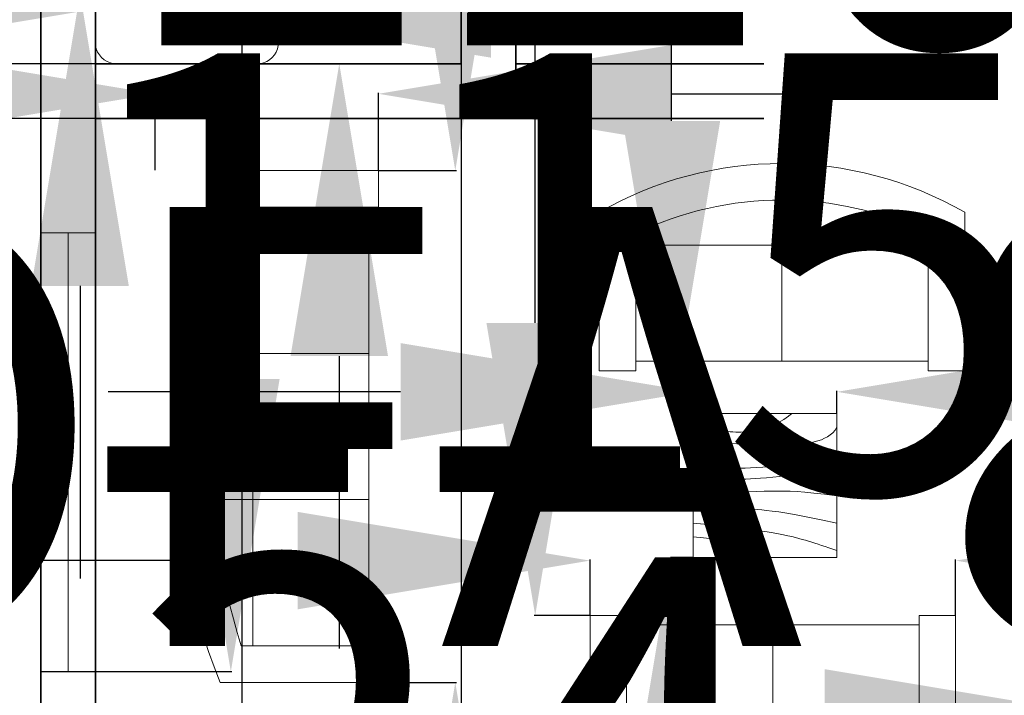
# Model space of a CAD drawing. Units: inches. Extents: x -307 to 2141, y -58 to 895.
# Tile 6 of 28: x 553 to 714, y 201 to 312. Entities that reach past the tile are written whole.
import ezdxf

# ---------------------------------------------------------------- set-up
doc = ezdxf.new("R2010")
doc.units = ezdxf.units.IN
doc.header["$MEASUREMENT"] = 0
for name, color, linetype, lineweight in [('A-ANNO-DIMS', 2, 'Continuous', 18), ('A-FURN', 8, 'Continuous', 18), ('A-GLAZ', 4, 'Continuous', 18), ('A-WALL', 7, 'Continuous', 35)]:
    doc.layers.add(name, color=color, linetype=linetype, lineweight=lineweight)
doc.styles.get("Standard").update_dxf_attribs({"font": 'arial.ttf'})
doc.dimstyles.get("Standard").update_dxf_attribs({"dimtxt": 72, "dimasz": 48, "dimexe": 0.18, "dimexo": 0.0625, "dimgap": 0.09, "dimtad": 0, "dimtih": 1, "dimtoh": 1, "dimdec": 0, "dimrnd": 48, "dimzin": 0, "dimdsep": 46, "dimlunit": 3, "dimtxsty": 'Standard', "dimcen": 0.09, "dimadec": 0, "dimazin": 0, "dimtfac": 1, "dimtdec": 0, "dimtofl": 0, "dimtmove": 0, "dimatfit": 3, "dimfxl": 1, "dimtolj": 1, "dimtzin": 0, "dimarcsym": 0})

# ---------------------------------------------------------------- blocks, each defined once
blk = doc.blocks.new('Desk - 30 x 60 in.')
for p, q in [((-26.999995, 0), (26.999995, 0)), ((-29.999995, -27), (-29.999995, -3)), ((29.999995, -3), (29.999995, -27)), ((26.999995, -30), (-26.999995, -30)), ((-20.000005, -30), (-20.000005, -31)), ((-16.000005, -31), (-16.000005, -30)), ((15.999995, -31), (15.999995, -30)), ((19.999995, -30), (19.999995, -31)), ((-20.000005, -31), (-16.000005, -31)), ((19.999995, -31), (15.999995, -31))]:
    blk.add_line(p, q)
for centre, start, end in [((-26.499995, -3.5), 98.1301, 171.8699), ((26.499995, -3.5), 8.130102, 81.8699), ((-26.499995, -26.5), 188.1301, 261.8699), ((26.499995, -26.5), 278.1301, 351.8699)]:
    blk.add_arc(centre, 3.535534, start, end)
blk = doc.blocks.new('Sofa - Roundback 7 ft.')
for p, q in [((-12.00002, -32.4421), (-12.00003, -6.5971)), ((11.99997, -32.4421), (11.99998, -6.5971)), ((-36.000027, -34), (-36.000027, -11.4696)), ((35.99998, -34), (35.99998, -11.4696)), ((-35.999844, -13.3819), (35.9998, -13.3819)), ((-36.000027, -32.4421), (35.99998, -32.4421))]:
    blk.add_line(p, q)
for points in [[(-36.000027, -34), (-42.000027, -34), (-42.000027, -8)], [(41.99998, -8), (41.99998, -34), (35.99998, -34)]]:
    blk.add_lwpolyline(points)
for centre, radius, start, end in [((0, -114.25), 114.25, 68.43141, 111.5686), ((-0.00001, -127.1968), 121.1968, 72.72033, 107.2797)]:
    blk.add_arc(centre, radius, start, end)
blk = doc.blocks.new('Sofa - Roundback Loveseat 5 ft.')
for p, q in [((0, -32.44198), (0, -5.99998)), ((-24, -33.99998), (-24, -11.46958)), ((24.00004, -33.99998), (24.00004, -11.46958)), ((-23.9998, -13.38178), (23.99986, -13.38178)), ((-24, -32.44198), (24.00004, -32.44198))]:
    blk.add_line(p, q)
for points in [[(-24, -33.99998), (-30, -33.99998), (-30, -7.99998)], [(30.00004, -7.99998), (30.00004, -33.99998), (24.00004, -33.99998)]]:
    blk.add_lwpolyline(points)
for centre, radius, start, end in [((0, -60.24998), 60.24998, 60.13715, 119.8628), ((0, -61.38438), 55.38444, 64.32083, 115.6792)]:
    blk.add_arc(centre, radius, start, end)
blk = doc.blocks.new('Table - Square Woodgrain 42 x 42 in.')
blk.add_line((0, -42), (42, -42))
for points in [[(0, -4), (1.704, -4.2172), (3.2358, -4.4188), (4.615, -4.604), (5.8615, -4.7721), (6.9951, -4.9224), (8.0357, -5.0541), (9.0031, -5.1667), (9.9171, -5.2594), (10.7951, -5.3316), (11.6445, -5.3836), (12.4702, -5.4157), (13.277, -5.4283), (14.0698, -5.4217), (14.8535, -5.3964), (15.6331, -5.3526), (16.4133, -5.2908), (17.1986, -5.2103), (17.9913, -5.1062), (18.793, -4.9727), (19.6056, -4.8038), (20.4307, -4.5937), (21.2701, -4.3365), (22.1256, -4.0262), (22.9989, -3.6571), (23.888, -3.2272), (24.7756, -2.7516), (25.6408, -2.2491), (26.4624, -1.7387), (27.2195, -1.2395), (27.891, -0.7703), (28.456, -0.3501), (28.8934, 0.002)], [(0, -42), (0, 0), (42, 0), (42, -42)], [(0, -8), (1.8203, -8.1001), (3.6741, -8.2149), (5.5411, -8.3408), (7.4011, -8.4741), (9.2339, -8.6112), (11.0193, -8.7484), (12.7371, -8.8821), (14.3671, -9.0086), (15.8954, -9.1246), (17.3337, -9.2278), (18.6997, -9.3159), (20.0116, -9.387), (21.2871, -9.4389), (22.5442, -9.4696), (23.8008, -9.477), (25.0749, -9.459), (26.3791, -9.4137), (27.7049, -9.3403), (29.0383, -9.2382), (30.3655, -9.1068), (31.6728, -8.9455), (32.9461, -8.7535), (34.1717, -8.5304), (35.3358, -8.2756), (36.4268, -7.9863), (37.443, -7.6521), (38.3849, -7.2603), (39.253, -6.7986), (40.048, -6.2542), (40.7705, -5.6147), (41.421, -4.8674), (42, -4)], [(42, -12), (39.1784, -12.8621), (36.4519, -13.5654), (33.8246, -14.1294), (31.3004, -14.5731), (28.8832, -14.9161), (26.577, -15.1775), (24.3858, -15.3768), (22.3136, -15.5332), (20.3622, -15.6632), (18.5254, -15.7718), (16.7947, -15.8612), (15.1618, -15.9338), (13.6183, -15.9916), (12.1558, -16.0369), (10.7659, -16.0718), (9.4403, -16.0987), (8.1703, -16.1191), (6.9461, -16.1325), (5.7577, -16.1377), (4.595, -16.1335), (3.4479, -16.1188), (2.3064, -16.0924), (1.1604, -16.0532), (0, -16)], [(42, -16), (37.6529, -16.7365), (33.8802, -17.329), (30.6179, -17.7961), (27.8015, -18.1561), (25.3668, -18.4275), (23.2497, -18.6288), (21.3859, -18.7785), (19.7111, -18.8949), (18.1693, -18.9939), (16.7375, -19.0795), (15.401, -19.1534), (14.1449, -19.217), (12.9544, -19.2717), (11.8148, -19.3191), (10.7113, -19.3606), (9.6291, -19.3976), (8.5534, -19.4323), (7.47, -19.4689), (6.3643, -19.5122), (5.222, -19.5672), (4.0288, -19.6386), (2.7703, -19.7313), (1.4321, -19.8501), (0, -20)], [(0, -24), (3.9243, -23.6805), (7.4766, -23.4138), (10.6891, -23.1954), (13.5943, -23.0205), (16.2247, -22.8847), (18.6125, -22.7832), (20.7903, -22.7116), (22.7903, -22.6651), (24.6563, -22.642), (26.4764, -22.6507), (28.35, -22.7024), (30.3766, -22.8084), (32.6555, -22.98), (35.2861, -23.2283), (38.3678, -23.5645), (42, -24)], [(42, -32), (37.392, -31.017), (33.4585, -30.2231), (30.1291, -29.5949), (27.3334, -29.109), (25.0009, -28.742), (23.0612, -28.4707), (21.4439, -28.2716), (20.0786, -28.1215), (18.8998, -28.0002), (17.8609, -27.9014), (16.9206, -27.8219), (16.0371, -27.7588), (15.1691, -27.709), (14.2748, -27.6693), (13.3128, -27.6368), (12.2415, -27.6083), (11.0295, -27.5824), (9.6867, -27.5643), (8.233, -27.5608), (6.6884, -27.5787), (5.0728, -27.6248), (3.4062, -27.7058), (1.7086, -27.8286), (0, -28)], [(0, -32), (5.4026, -32.5358), (9.9494, -33.019), (13.7424, -33.4553), (16.8834, -33.8505), (19.4743, -34.2106), (21.6171, -34.5413), (23.4136, -34.8486), (24.9657, -35.1382), (26.3614, -35.4156), (27.6332, -35.6841), (28.7995, -35.9467), (29.8788, -36.2064), (30.8897, -36.4661), (31.8507, -36.7288), (32.7802, -36.9973), (33.6968, -37.2747), (34.6175, -37.5635), (35.5531, -37.8651), (36.5128, -38.1805), (37.506, -38.5108), (38.5421, -38.8568), (39.6302, -39.2197), (40.7797, -39.6004), (42, -40)], [(0, -36), (3.0098, -36.2857), (5.5354, -36.5643), (7.6368, -36.8359), (9.374, -37.1009), (10.807, -37.3597), (11.9957, -37.6126), (13.0002, -37.8599), (13.8804, -38.102), (14.6874, -38.3393), (15.4365, -38.5729), (16.1338, -38.8041), (16.7858, -39.0341), (17.3987, -39.264), (17.9787, -39.4952), (18.5322, -39.7288), (19.0655, -39.9662), (19.5832, -40.2081), (20.0842, -40.4544), (20.5657, -40.7046), (21.0249, -40.9581), (21.459, -41.2144), (21.8653, -41.4731), (22.2409, -41.7335), (22.5831, -41.9951)]]:
    blk.add_lwpolyline(points)
blk = doc.blocks.new('WIN-72IN')
blk.add_line((72, 4.5), (0, 4.5))
blk.add_lwpolyline([(72, 0), (0, 0), (0, 9), (72, 9)], close=True)
blk = doc.blocks.new('*D28')
at = {"layer": 'A-ANNO-DIMS', "color": 0, "lineweight": -2, "transparency": 16777216}
for p, q in [((795.36, 433.55), (777.92, 433.55)), ((778.1, 385.55), (778.1, 366.07)), ((795.36, 318.07), (777.92, 318.07)), ((778.1, 318.07), (778.1, 270.07)), ((778.1, 270.07), (730.1, 270.07))]:
    blk.add_line(p, q, dxfattribs=at)
at = {"layer": 'A-ANNO-DIMS', "color": 0, "transparency": 16777216}
for points in [[(770.1, 385.55), (786.1, 385.55), (778.1, 433.55)], [(770.1, 366.07), (786.1, 366.07), (778.1, 318.07)]]:
    blk.add_solid(points, dxfattribs=at)
at = {"layer": 'Defpoints', "color": 0, "transparency": 16777216}
for p in [(795.42, 433.55), (778.1, 318.07), (795.42, 318.07)]:
    blk.add_point(p, dxfattribs=at)
at = {"layer": 'A-ANNO-DIMS', "color": 0, "transparency": 16777216, "insert": (534.42, 270.07), "char_height": 72, "attachment_point": 5}
blk.add_mtext('\\A1;BED 115', dxfattribs=at)
blk = doc.blocks.new('*D36')
at = {"layer": 'A-ANNO-DIMS', "color": 0, "lineweight": -2, "transparency": 16777216}
for p, q in [((871.71, 562.4), (871.76, 610.4)), ((876.55, 514.4), (871.47, 514.4)), ((876.51, 481.35), (871.44, 481.36)), ((871.56, 433.36), (871.51, 385.36)), ((871.51, 385.36), (823.51, 385.36))]:
    blk.add_line(p, q, dxfattribs=at)
at = {"layer": 'A-ANNO-DIMS', "color": 0, "transparency": 16777216}
for points in [[(863.71, 562.41), (879.71, 562.4), (871.65, 514.4)], [(863.56, 433.37), (879.56, 433.35), (871.62, 481.36)]]:
    blk.add_solid(points, dxfattribs=at)
at = {"layer": 'Defpoints', "color": 0, "transparency": 16777216}
for p in [(876.61, 514.4), (871.62, 481.36), (876.57, 481.35)]:
    blk.add_point(p, dxfattribs=at)
at = {"layer": 'A-ANNO-DIMS', "color": 0, "transparency": 16777216, "insert": (548.95, 385.36), "char_height": 72, "attachment_point": 5}
blk.add_mtext('\\A1;WC 33 TYP.', dxfattribs=at)
blk = doc.blocks.new('*D38')
at = {"layer": 'A-ANNO-DIMS', "color": 0, "lineweight": -2, "transparency": 16777216}
for p, q in [((598.5, 222.79), (550.5, 222.79)), ((646.5, 213.85), (646.5, 222.97)), ((706.5, 213.85), (706.5, 222.97)), ((754.5, 222.79), (802.5, 222.79))]:
    blk.add_line(p, q, dxfattribs=at)
at = {"layer": 'A-ANNO-DIMS', "color": 0, "transparency": 16777216}
for points in [[(598.5, 230.79), (598.5, 214.79), (646.5, 222.79)], [(754.5, 230.79), (754.5, 214.79), (706.5, 222.79)]]:
    blk.add_solid(points, dxfattribs=at)
at = {"layer": 'Defpoints', "color": 0, "transparency": 16777216}
for p in [(646.5, 222.79), (646.5, 213.79), (706.5, 213.79)]:
    blk.add_point(p, dxfattribs=at)
at = {"layer": 'A-ANNO-DIMS', "color": 0, "transparency": 16777216, "insert": (97.26, 222.79), "char_height": 72, "attachment_point": 5}
blk.add_mtext('\\A1;LOVESEAT 60 TYP.', dxfattribs=at)
blk = doc.blocks.new('*D39')
at = {"layer": 'A-ANNO-DIMS', "color": 0, "lineweight": -2, "transparency": 16777216}
for p, q in [((637.5, 261.79), (637.5, 309.79)), ((646.43, 213.79), (637.32, 213.79)), ((646.43, 177.12), (637.32, 177.12)), ((637.5, 129.12), (637.5, 81.12)), ((637.5, 81.12), (589.5, 81.12))]:
    blk.add_line(p, q, dxfattribs=at)
at = {"layer": 'A-ANNO-DIMS', "color": 0, "transparency": 16777216}
for points in [[(629.5, 261.79), (645.5, 261.79), (637.5, 213.79)], [(629.5, 129.12), (645.5, 129.12), (637.5, 177.12)]]:
    blk.add_solid(points, dxfattribs=at)
at = {"layer": 'Defpoints', "color": 0, "transparency": 16777216}
for p in [(646.5, 213.79), (637.5, 177.12), (646.5, 177.12)]:
    blk.add_point(p, dxfattribs=at)
at = {"layer": 'A-ANNO-DIMS', "color": 0, "transparency": 16777216, "insert": (414.2, 81.12), "char_height": 72, "attachment_point": 5}
blk.add_mtext('\\A1;37 TYP.', dxfattribs=at)
blk = doc.blocks.new('*D40')
at = {"layer": 'A-ANNO-DIMS', "color": 0, "lineweight": -2, "transparency": 16777216}
for p, q in [((725.38, 128.89), (725.38, 123.17)), ((762.77, 128.89), (762.77, 123.17)), ((677.38, 123.35), (629.38, 123.35)), ((810.77, 123.35), (858.77, 123.35))]:
    blk.add_line(p, q, dxfattribs=at)
at = {"layer": 'A-ANNO-DIMS', "color": 0, "transparency": 16777216}
for points in [[(677.38, 131.35), (677.38, 115.35), (725.38, 123.35)], [(810.77, 131.35), (810.77, 115.35), (762.77, 123.35)]]:
    blk.add_solid(points, dxfattribs=at)
at = {"layer": 'Defpoints', "color": 0, "transparency": 16777216}
for p in [(725.38, 128.96), (762.77, 128.96), (762.77, 123.35)]:
    blk.add_point(p, dxfattribs=at)
at = {"layer": 'A-ANNO-DIMS', "color": 0, "transparency": 16777216, "insert": (1208.37, 123.35), "char_height": 72, "attachment_point": 5}
blk.add_mtext('\\A1;PLANT 37 TYP.', dxfattribs=at)
blk = doc.blocks.new('*D48')
at = {"layer": 'A-ANNO-DIMS', "color": 0, "lineweight": -2, "transparency": 16777216}
for p, q in [((724, 313.98), (724, 361.98)), ((732.94, 265.98), (723.82, 265.98)), ((732.94, 205.98), (723.82, 205.98)), ((724, 157.98), (724, 109.98)), ((724, 109.98), (676, 109.98))]:
    blk.add_line(p, q, dxfattribs=at)
at = {"layer": 'A-ANNO-DIMS', "color": 0, "transparency": 16777216}
for points in [[(716, 313.98), (732, 313.98), (724, 265.98)], [(716, 157.98), (732, 157.98), (724, 205.98)]]:
    blk.add_solid(points, dxfattribs=at)
at = {"layer": 'Defpoints', "color": 0, "transparency": 16777216}
for p in [(733, 265.98), (724, 205.98), (733, 205.98)]:
    blk.add_point(p, dxfattribs=at)
at = {"layer": 'A-ANNO-DIMS', "color": 0, "transparency": 16777216, "insert": (321.56, 109.98), "char_height": 72, "attachment_point": 5}
blk.add_mtext('\\A1;MEDIA UNIT 60', dxfattribs=at)
blk = doc.blocks.new('*D49')
at = {"layer": 'A-ANNO-DIMS', "color": 0, "lineweight": -2, "transparency": 16777216}
for p, q in [((733, 205.92), (733, 196.8)), ((754.34, 205.92), (754.34, 196.8)), ((685, 196.98), (637, 196.98)), ((802.34, 196.98), (850.34, 196.98))]:
    blk.add_line(p, q, dxfattribs=at)
at = {"layer": 'A-ANNO-DIMS', "color": 0, "transparency": 16777216}
for points in [[(685, 204.98), (685, 188.98), (733, 196.98)], [(802.34, 204.98), (802.34, 188.98), (754.34, 196.98)]]:
    blk.add_solid(points, dxfattribs=at)
at = {"layer": 'Defpoints', "color": 0, "transparency": 16777216}
for p in [(733, 205.98), (754.34, 205.98), (754.34, 196.98)]:
    blk.add_point(p, dxfattribs=at)
at = {"layer": 'A-ANNO-DIMS', "color": 0, "transparency": 16777216, "insert": (895.66, 196.98), "char_height": 72, "attachment_point": 5}
blk.add_mtext('\\A1;21', dxfattribs=at)
blk = doc.blocks.new('*D50')
at = {"layer": 'A-ANNO-DIMS', "color": 0, "lineweight": -2, "transparency": 16777216}
for p, q in [((565.34, 315.8), (565.34, 313.15)), ((582.27, 315.8), (582.27, 313.15)), ((517.34, 313.33), (469.34, 313.33)), ((630.27, 313.33), (678.27, 313.33))]:
    blk.add_line(p, q, dxfattribs=at)
at = {"layer": 'A-ANNO-DIMS', "color": 0, "transparency": 16777216}
for points in [[(517.34, 321.33), (517.34, 305.33), (565.34, 313.33)], [(630.27, 321.33), (630.27, 305.33), (582.27, 313.33)]]:
    blk.add_solid(points, dxfattribs=at)
at = {"layer": 'Defpoints', "color": 0, "transparency": 16777216}
for p in [(565.34, 315.87), (582.27, 315.87), (565.34, 313.33)]:
    blk.add_point(p, dxfattribs=at)
at = {"layer": 'A-ANNO-DIMS', "color": 0, "transparency": 16777216, "insert": (226.65, 313.33), "char_height": 72, "attachment_point": 5}
blk.add_mtext('\\A1;PHONE 17', dxfattribs=at)
blk = doc.blocks.new('*D51')
at = {"layer": 'A-ANNO-DIMS', "color": 0, "lineweight": -2, "transparency": 16777216}
for p, q in [((562.8, 379.11), (562.8, 427.11)), ((562.8, 427.11), (610.8, 427.11)), ((565.27, 331.11), (562.62, 331.11)), ((565.27, 315.87), (562.62, 315.87)), ((562.8, 267.87), (562.8, 219.87))]:
    blk.add_line(p, q, dxfattribs=at)
at = {"layer": 'A-ANNO-DIMS', "color": 0, "transparency": 16777216}
for points in [[(554.8, 379.11), (570.8, 379.11), (562.8, 331.11)], [(554.8, 267.87), (570.8, 267.87), (562.8, 315.87)]]:
    blk.add_solid(points, dxfattribs=at)
at = {"layer": 'Defpoints', "color": 0, "transparency": 16777216}
for p in [(562.8, 331.11), (565.34, 331.11), (565.34, 315.87)]:
    blk.add_point(p, dxfattribs=at)
at = {"layer": 'A-ANNO-DIMS', "color": 0, "transparency": 16777216, "insert": (659.34, 427.11), "char_height": 72, "attachment_point": 5}
blk.add_mtext('\\A1;15', dxfattribs=at)
blk = doc.blocks.new('*D52')
at = {"layer": 'A-ANNO-DIMS', "color": 0, "lineweight": -2, "transparency": 16777216}
for p, q in [((660.21, 554.25), (660.21, 602.25)), ((673.8, 506.25), (660.03, 506.25)), ((673.8, 415.25), (660.03, 415.25)), ((660.21, 367.25), (660.21, 319.25))]:
    blk.add_line(p, q, dxfattribs=at)
at = {"layer": 'A-ANNO-DIMS', "color": 0, "transparency": 16777216}
for points in [[(652.21, 554.25), (668.21, 554.25), (660.21, 506.25)], [(652.21, 367.25), (668.21, 367.25), (660.21, 415.25)]]:
    blk.add_solid(points, dxfattribs=at)
at = {"layer": 'Defpoints', "color": 0, "transparency": 16777216}
for p in [(673.86, 506.25), (660.21, 415.25), (673.86, 415.25)]:
    blk.add_point(p, dxfattribs=at)
at = {"layer": 'A-ANNO-DIMS', "color": 0, "transparency": 16777216, "insert": (660.21, 460.75), "char_height": 72, "attachment_point": 5}
blk.add_mtext('\\A1;DINING SET 91', dxfattribs=at)
blk = doc.blocks.new('*D54')
at = {"layer": 'A-ANNO-DIMS', "color": 0, "lineweight": -2, "transparency": 16777216}
for p, q in [((605.34, 412.35), (605.34, 460.35)), ((605.34, 460.35), (653.34, 460.35)), ((596.4, 364.35), (605.52, 364.35)), ((596.4, 304.35), (605.52, 304.35)), ((605.34, 256.35), (605.34, 208.35))]:
    blk.add_line(p, q, dxfattribs=at)
at = {"layer": 'A-ANNO-DIMS', "color": 0, "transparency": 16777216}
for points in [[(597.34, 412.35), (613.34, 412.35), (605.34, 364.35)], [(597.34, 256.35), (613.34, 256.35), (605.34, 304.35)]]:
    blk.add_solid(points, dxfattribs=at)
at = {"layer": 'Defpoints', "color": 0, "transparency": 16777216}
for p in [(596.34, 364.35), (605.34, 364.35), (596.34, 304.35)]:
    blk.add_point(p, dxfattribs=at)
at = {"layer": 'A-ANNO-DIMS', "color": 0, "transparency": 16777216, "insert": (854, 460.35), "char_height": 72, "attachment_point": 5}
blk.add_mtext('\\A1;DESK 60', dxfattribs=at)
blk = doc.blocks.new('*D58')
at = {"layer": 'A-ANNO-DIMS', "color": 0, "lineweight": -2, "transparency": 16777216}
for p, q in [((624.38, 334.8), (624.38, 382.8)), ((611.84, 286.8), (624.56, 286.8)), ((611.84, 202.8), (624.56, 202.8)), ((624.38, 154.8), (624.38, 106.8))]:
    blk.add_line(p, q, dxfattribs=at)
at = {"layer": 'A-ANNO-DIMS', "color": 0, "transparency": 16777216}
for points in [[(616.38, 334.8), (632.38, 334.8), (624.38, 286.8)], [(616.38, 154.8), (632.38, 154.8), (624.38, 202.8)]]:
    blk.add_solid(points, dxfattribs=at)
at = {"layer": 'Defpoints', "color": 0, "transparency": 16777216}
for p in [(611.78, 286.8), (624.38, 286.8), (611.78, 202.8)]:
    blk.add_point(p, dxfattribs=at)
at = {"layer": 'A-ANNO-DIMS', "color": 0, "transparency": 16777216, "insert": (624.38, 244.8), "char_height": 72, "attachment_point": 5}
blk.add_mtext('\\A1;SOFA 84', dxfattribs=at)
blk = doc.blocks.new('*D59')
at = {"layer": 'A-ANNO-DIMS', "color": 0, "lineweight": -2, "transparency": 16777216}
for p, q in [((527.11, 299.4), (479.11, 299.4)), ((575.11, 286.86), (575.11, 299.58)), ((611.78, 286.86), (611.78, 299.58)), ((659.78, 299.4), (707.78, 299.4))]:
    blk.add_line(p, q, dxfattribs=at)
at = {"layer": 'A-ANNO-DIMS', "color": 0, "transparency": 16777216}
for points in [[(527.11, 307.4), (527.11, 291.4), (575.11, 299.4)], [(659.78, 307.4), (659.78, 291.4), (611.78, 299.4)]]:
    blk.add_solid(points, dxfattribs=at)
at = {"layer": 'Defpoints', "color": 0, "transparency": 16777216}
for p in [(575.11, 299.4), (575.11, 286.8), (611.78, 286.8)]:
    blk.add_point(p, dxfattribs=at)
at = {"layer": 'A-ANNO-DIMS', "color": 0, "transparency": 16777216, "insert": (427.48, 299.4), "char_height": 72, "attachment_point": 5}
blk.add_mtext('\\A1;37', dxfattribs=at)
blk = doc.blocks.new('*D60')
at = {"layer": 'A-ANNO-DIMS', "color": 0, "lineweight": -2, "transparency": 16777216}
for p, q in [((659.86, 294.95), (659.86, 342.95)), ((659.86, 342.95), (707.86, 342.95)), ((663.34, 246.95), (659.68, 246.95)), ((663.34, 223.32), (659.68, 223.32)), ((659.86, 175.32), (659.86, 127.32))]:
    blk.add_line(p, q, dxfattribs=at)
at = {"layer": 'A-ANNO-DIMS', "color": 0, "transparency": 16777216}
for points in [[(651.86, 294.95), (667.86, 294.95), (659.86, 246.95)], [(651.86, 175.32), (667.86, 175.32), (659.86, 223.32)]]:
    blk.add_solid(points, dxfattribs=at)
at = {"layer": 'Defpoints', "color": 0, "transparency": 16777216}
for p in [(659.86, 246.95), (663.4, 246.95), (663.4, 223.32)]:
    blk.add_point(p, dxfattribs=at)
at = {"layer": 'A-ANNO-DIMS', "color": 0, "transparency": 16777216, "insert": (933.57, 342.95), "char_height": 72, "attachment_point": 5}
blk.add_mtext('\\A1;TABLE 24', dxfattribs=at)
blk = doc.blocks.new('*D61')
at = {"layer": 'A-ANNO-DIMS', "color": 0, "lineweight": -2, "transparency": 16777216}
for p, q in [((615.4, 250.49), (567.4, 250.49)), ((663.4, 247.01), (663.4, 250.67)), ((687.03, 247.01), (687.03, 250.67)), ((735.03, 250.49), (783.03, 250.49))]:
    blk.add_line(p, q, dxfattribs=at)
at = {"layer": 'A-ANNO-DIMS', "color": 0, "transparency": 16777216}
for points in [[(615.4, 258.49), (615.4, 242.49), (663.4, 250.49)], [(735.03, 258.49), (735.03, 242.49), (687.03, 250.49)]]:
    blk.add_solid(points, dxfattribs=at)
at = {"layer": 'Defpoints', "color": 0, "transparency": 16777216}
for p in [(687.03, 250.49), (663.4, 246.95), (687.03, 246.95)]:
    blk.add_point(p, dxfattribs=at)
at = {"layer": 'A-ANNO-DIMS', "color": 0, "transparency": 16777216, "insert": (835.16, 250.49), "char_height": 72, "attachment_point": 5}
blk.add_mtext('\\A1;24', dxfattribs=at)
blk = doc.blocks.new('*D63')
at = {"layer": 'A-ANNO-DIMS', "color": 0, "lineweight": -2, "transparency": 16777216}
for p, q in [((916.4, 691.34), (947.72, 691.34)), ((947.54, 643.34), (947.54, 416.19)), ((947.54, 115.34), (947.54, 342.49)), ((704.68, 67.34), (947.72, 67.34))]:
    blk.add_line(p, q, dxfattribs=at)
at = {"layer": 'A-ANNO-DIMS', "color": 0, "transparency": 16777216}
for points in [[(939.54, 643.34), (955.54, 643.34), (947.54, 691.34)], [(939.54, 115.34), (955.54, 115.34), (947.54, 67.34)]]:
    blk.add_solid(points, dxfattribs=at)
at = {"layer": 'Defpoints', "color": 0, "transparency": 16777216}
for p in [(916.34, 691.34), (704.62, 67.34), (947.54, 67.34)]:
    blk.add_point(p, dxfattribs=at)
at = {"layer": 'A-ANNO-DIMS', "color": 0, "transparency": 16777216, "insert": (947.54, 379.34), "char_height": 72, "attachment_point": 5}
blk.add_mtext('\\A1;624', dxfattribs=at)
blk = doc.blocks.new('*D64')
at = {"layer": 'A-ANNO-DIMS', "color": 0, "lineweight": -2, "transparency": 16777216}
for p, q in [((556.27, 691.34), (524.95, 691.34)), ((525.13, 643.34), (525.13, 465.69)), ((525.13, 214.34), (525.13, 391.99)), ((556.27, 166.34), (524.95, 166.34))]:
    blk.add_line(p, q, dxfattribs=at)
at = {"layer": 'A-ANNO-DIMS', "color": 0, "transparency": 16777216}
for points in [[(517.13, 643.34), (533.13, 643.34), (525.13, 691.34)], [(517.13, 214.34), (533.13, 214.34), (525.13, 166.34)]]:
    blk.add_solid(points, dxfattribs=at)
at = {"layer": 'Defpoints', "color": 0, "transparency": 16777216}
for p in [(525.13, 691.34), (556.34, 691.34), (556.34, 166.34)]:
    blk.add_point(p, dxfattribs=at)
at = {"layer": 'A-ANNO-DIMS', "color": 0, "transparency": 16777216, "insert": (525.13, 428.84), "char_height": 72, "attachment_point": 5}
blk.add_mtext('\\A1;525', dxfattribs=at)
blk = doc.blocks.new('*D65')
at = {"layer": 'A-ANNO-DIMS', "color": 0, "lineweight": -2, "transparency": 16777216}
for p, q in [((587.54, 252.57), (587.54, 300.57)), ((556.4, 204.57), (587.72, 204.57)), ((556.4, 166.34), (587.72, 166.34)), ((587.54, 118.34), (587.54, 70.34)), ((587.54, 70.34), (539.54, 70.34))]:
    blk.add_line(p, q, dxfattribs=at)
at = {"layer": 'A-ANNO-DIMS', "color": 0, "transparency": 16777216}
for points in [[(579.54, 252.57), (595.54, 252.57), (587.54, 204.57)], [(579.54, 118.34), (595.54, 118.34), (587.54, 166.34)]]:
    blk.add_solid(points, dxfattribs=at)
at = {"layer": 'Defpoints', "color": 0, "transparency": 16777216}
for p in [(556.34, 204.57), (556.34, 166.34), (587.54, 166.34)]:
    blk.add_point(p, dxfattribs=at)
at = {"layer": 'A-ANNO-DIMS', "color": 0, "transparency": 16777216, "insert": (417.99, 70.34), "char_height": 72, "attachment_point": 5}
blk.add_mtext('\\A1;38.23', dxfattribs=at)
blk = doc.blocks.new('*D66')
at = {"layer": 'A-ANNO-DIMS', "color": 0, "lineweight": -2, "transparency": 16777216}
for p, q in [((525.13, 382.34), (525.13, 430.34)), ((556.27, 334.34), (524.95, 334.34)), ((565.27, 304.34), (524.95, 304.34)), ((525.13, 256.34), (525.13, 208.34)), ((525.13, 208.34), (477.13, 208.34))]:
    blk.add_line(p, q, dxfattribs=at)
at = {"layer": 'A-ANNO-DIMS', "color": 0, "transparency": 16777216}
for points in [[(517.13, 382.34), (533.13, 382.34), (525.13, 334.34)], [(517.13, 256.34), (533.13, 256.34), (525.13, 304.34)]]:
    blk.add_solid(points, dxfattribs=at)
at = {"layer": 'Defpoints', "color": 0, "transparency": 16777216}
for p in [(556.34, 334.34), (525.13, 304.34), (565.34, 304.34)]:
    blk.add_point(p, dxfattribs=at)
at = {"layer": 'A-ANNO-DIMS', "color": 0, "transparency": 16777216, "insert": (425.62, 208.34), "char_height": 72, "attachment_point": 5}
blk.add_mtext('\\A1;30', dxfattribs=at)
blk = doc.blocks.new('*D67')
at = {"layer": 'A-ANNO-DIMS', "color": 0, "lineweight": -2, "transparency": 16777216}
for p, q in [((525.13, 496.83), (525.13, 544.83)), ((556.27, 448.83), (524.95, 448.83)), ((556.27, 370.34), (524.95, 370.34)), ((525.13, 322.34), (525.13, 274.34))]:
    blk.add_line(p, q, dxfattribs=at)
at = {"layer": 'A-ANNO-DIMS', "color": 0, "transparency": 16777216}
for points in [[(517.13, 496.83), (533.13, 496.83), (525.13, 448.83)], [(517.13, 322.34), (533.13, 322.34), (525.13, 370.34)]]:
    blk.add_solid(points, dxfattribs=at)
at = {"layer": 'Defpoints', "color": 0, "transparency": 16777216}
for p in [(525.13, 448.83), (556.34, 448.83), (556.34, 370.34)]:
    blk.add_point(p, dxfattribs=at)
at = {"layer": 'A-ANNO-DIMS', "color": 0, "transparency": 16777216, "insert": (525.13, 409.59), "char_height": 72, "attachment_point": 5}
blk.add_mtext('\\A1;78.49', dxfattribs=at)
blk = doc.blocks.new('*D70')
at = {"layer": 'A-ANNO-DIMS', "color": 0, "lineweight": -2, "transparency": 16777216}
for p, q in [((525.13184, 214.340828), (525.13184, 262.340828)), ((556.27334, 166.340828), (524.95184, 166.340828)), ((556.27334, 91.340828), (524.95184, 91.340828)), ((525.13184, 43.340828), (525.13184, -4.659172))]:
    blk.add_line(p, q, dxfattribs=at)
at = {"layer": 'A-ANNO-DIMS', "color": 0, "transparency": 16777216}
for points in [[(517.13184, 214.340828), (533.13184, 214.340828), (525.13184, 166.340828)], [(517.13184, 43.340828), (533.13184, 43.340828), (525.13184, 91.340828)]]:
    blk.add_solid(points, dxfattribs=at)
at = {"layer": 'Defpoints', "color": 0, "transparency": 16777216}
for p in [(525.13184, 166.340828), (556.33584, 166.340828), (556.33584, 91.340828)]:
    blk.add_point(p, dxfattribs=at)
at = {"layer": 'A-ANNO-DIMS', "color": 0, "transparency": 16777216, "insert": (525.13184, 128.840828), "char_height": 72, "attachment_point": 5}
blk.add_mtext('\\A1;75', dxfattribs=at)
blk = doc.blocks.new('*D71')
at = {"layer": 'A-ANNO-DIMS', "color": 0, "lineweight": -2, "transparency": 16777216}
for p, q in [((525.13, 139.34), (525.13, 187.34)), ((525.13, 187.34), (573.13, 187.34)), ((632.56, 91.34), (524.95, 91.34)), ((632.56, 67.34), (524.95, 67.34)), ((525.13, 19.34), (525.13, -28.66))]:
    blk.add_line(p, q, dxfattribs=at)
at = {"layer": 'A-ANNO-DIMS', "color": 0, "transparency": 16777216}
for points in [[(517.13, 139.34), (533.13, 139.34), (525.13, 91.34)], [(517.13, 19.34), (533.13, 19.34), (525.13, 67.34)]]:
    blk.add_solid(points, dxfattribs=at)
at = {"layer": 'Defpoints', "color": 0, "transparency": 16777216}
for p in [(525.13, 91.34), (632.62, 91.34), (632.62, 67.34)]:
    blk.add_point(p, dxfattribs=at)
at = {"layer": 'A-ANNO-DIMS', "color": 0, "transparency": 16777216, "insert": (625.26, 187.34), "char_height": 72, "attachment_point": 5}
blk.add_mtext('\\A1;24', dxfattribs=at)
blk = doc.blocks.new('*D86')
at = {"layer": 'A-ANNO-DIMS', "color": 0, "lineweight": -2, "transparency": 16777216}
for p, q in [((565.34, 304.28), (565.34, 35.96)), ((625.34, 304.28), (625.34, 35.96)), ((517.34, 36.14), (469.34, 36.14)), ((673.34, 36.14), (721.34, 36.14))]:
    blk.add_line(p, q, dxfattribs=at)
at = {"layer": 'A-ANNO-DIMS', "color": 0, "transparency": 16777216}
for points in [[(517.34, 44.14), (517.34, 28.14), (565.34, 36.14)], [(673.34, 44.14), (673.34, 28.14), (625.34, 36.14)]]:
    blk.add_solid(points, dxfattribs=at)
at = {"layer": 'Defpoints', "color": 0, "transparency": 16777216}
for p in [(565.34, 304.34), (625.34, 304.34), (625.34, 36.14)]:
    blk.add_point(p, dxfattribs=at)
at = {"layer": 'A-ANNO-DIMS', "color": 0, "transparency": 16777216, "insert": (773.07, 36.14), "char_height": 72, "attachment_point": 5}
blk.add_mtext('\\A1;60', dxfattribs=at)
blk = doc.blocks.new('*D87')
at = {"layer": 'A-ANNO-DIMS', "color": 0, "lineweight": -2, "transparency": 16777216}
for p, q in [((525.13184, 448.340828), (525.13184, 496.340828)), ((625.27334, 400.340828), (524.95184, 400.340828)), ((625.27334, 304.340828), (524.95184, 304.340828)), ((525.13184, 256.340828), (525.13184, 208.340828))]:
    blk.add_line(p, q, dxfattribs=at)
at = {"layer": 'A-ANNO-DIMS', "color": 0, "transparency": 16777216}
for points in [[(517.13184, 448.340828), (533.13184, 448.340828), (525.13184, 400.340828)], [(517.13184, 256.340828), (533.13184, 256.340828), (525.13184, 304.340828)]]:
    blk.add_solid(points, dxfattribs=at)
at = {"layer": 'Defpoints', "color": 0, "transparency": 16777216}
for p in [(525.13184, 400.340828), (625.33584, 400.340828), (625.33584, 304.340828)]:
    blk.add_point(p, dxfattribs=at)
at = {"layer": 'A-ANNO-DIMS', "color": 0, "transparency": 16777216, "insert": (525.13184, 352.340828), "char_height": 72, "attachment_point": 5}
blk.add_mtext('\\A1;96', dxfattribs=at)
blk = doc.blocks.new('*D88')
at = {"layer": 'A-ANNO-DIMS', "color": 0, "lineweight": -2, "transparency": 16777216}
for p, q in [((517.33584, 722.544828), (469.33584, 722.544828)), ((565.33584, 295.403328), (565.33584, 722.724828)), ((754.33584, 271.403328), (754.33584, 722.724828)), ((802.33584, 722.544828), (850.33584, 722.544828))]:
    blk.add_line(p, q, dxfattribs=at)
at = {"layer": 'A-ANNO-DIMS', "color": 0, "transparency": 16777216}
for points in [[(517.33584, 730.544828), (517.33584, 714.544828), (565.33584, 722.544828)], [(802.33584, 730.544828), (802.33584, 714.544828), (754.33584, 722.544828)]]:
    blk.add_solid(points, dxfattribs=at)
at = {"layer": 'Defpoints', "color": 0, "transparency": 16777216}
for p in [(754.33584, 722.544828), (565.33584, 295.340828), (754.33584, 271.340828)]:
    blk.add_point(p, dxfattribs=at)
at = {"layer": 'A-ANNO-DIMS', "color": 0, "transparency": 16777216, "insert": (659.83584, 722.544828), "char_height": 72, "attachment_point": 5}
blk.add_mtext('\\A1;189', dxfattribs=at)
blk = doc.blocks.new('*D89')
at = {"layer": 'A-ANNO-DIMS', "color": 0, "lineweight": -2, "transparency": 16777216}
for p, q in [((525.13, 295.34), (525.13, 343.34)), ((525.13, 343.34), (573.13, 343.34)), ((565.27, 295.34), (524.95, 295.34)), ((525.13, 223.34), (525.13, 247.34)), ((556.27, 175.34), (524.95, 175.34))]:
    blk.add_line(p, q, dxfattribs=at)
at = {"layer": 'A-ANNO-DIMS', "color": 0, "transparency": 16777216}
for points in [[(517.13, 247.34), (533.13, 247.34), (525.13, 295.34)], [(517.13, 223.34), (533.13, 223.34), (525.13, 175.34)]]:
    blk.add_solid(points, dxfattribs=at)
at = {"layer": 'Defpoints', "color": 0, "transparency": 16777216}
for p in [(525.13, 295.34), (565.34, 295.34), (556.34, 175.34)]:
    blk.add_point(p, dxfattribs=at)
at = {"layer": 'A-ANNO-DIMS', "color": 0, "transparency": 16777216, "insert": (649.25, 343.34), "char_height": 72, "attachment_point": 5}
blk.add_mtext('\\A1;120', dxfattribs=at)
blk = doc.blocks.new('*D99')
at = {"layer": 'A-ANNO-DIMS', "color": 0, "lineweight": -2, "transparency": 16777216}
for p, q in [((763.34, 481.28), (763.34, 35.96)), ((802.34, 481.28), (802.34, 35.96)), ((715.34, 36.14), (667.34, 36.14)), ((850.34, 36.14), (898.34, 36.14))]:
    blk.add_line(p, q, dxfattribs=at)
at = {"layer": 'A-ANNO-DIMS', "color": 0, "transparency": 16777216}
for points in [[(715.34, 44.14), (715.34, 28.14), (763.34, 36.14)], [(850.34, 44.14), (850.34, 28.14), (802.34, 36.14)]]:
    blk.add_solid(points, dxfattribs=at)
at = {"layer": 'Defpoints', "color": 0, "transparency": 16777216}
for p in [(763.34, 481.34), (802.34, 481.34), (802.34, 36.14)]:
    blk.add_point(p, dxfattribs=at)
at = {"layer": 'A-ANNO-DIMS', "color": 0, "transparency": 16777216, "insert": (950.04, 36.14), "char_height": 72, "attachment_point": 5}
blk.add_mtext('\\A1;39', dxfattribs=at)
blk = doc.blocks.new('*D100')
at = {"layer": 'A-ANNO-DIMS', "color": 0, "lineweight": -2, "transparency": 16777216}
for p, q in [((589.34, 409.28), (589.34, 35.96)), ((625.34, 409.28), (625.34, 35.96)), ((541.34, 36.14), (493.34, 36.14)), ((673.34, 36.14), (721.34, 36.14))]:
    blk.add_line(p, q, dxfattribs=at)
at = {"layer": 'A-ANNO-DIMS', "color": 0, "transparency": 16777216}
for points in [[(541.34, 44.14), (541.34, 28.14), (589.34, 36.14)], [(673.34, 44.14), (673.34, 28.14), (625.34, 36.14)]]:
    blk.add_solid(points, dxfattribs=at)
at = {"layer": 'Defpoints', "color": 0, "transparency": 16777216}
for p in [(589.34, 409.34), (625.34, 409.34), (625.34, 36.14)]:
    blk.add_point(p, dxfattribs=at)
at = {"layer": 'A-ANNO-DIMS', "color": 0, "transparency": 16777216, "insert": (772.95, 36.14), "char_height": 72, "attachment_point": 5}
blk.add_mtext('\\A1;36', dxfattribs=at)

msp = doc.modelspace()

# ---------------------------------------------------------------- linework, layer by layer
at = {"layer": 'A-WALL'}
for p, q in [((556.3358, 691.3408), (556.3358, 91.3408)), ((565.3358, 682.3408), (565.3358, 100.3408)), ((625.3358, 400.3408), (625.3358, 304.3408)), ((634.3358, 400.3408), (634.3358, 295.3408)), ((625.3358, 304.3408), (565.3358, 304.3408)), ((634.3358, 304.3408), (675.0316, 304.3408)), ((634.3358, 295.3408), (565.3358, 295.3408)), ((634.3358, 295.3408), (675.0316, 295.3408))]:
    msp.add_line(p, q, dxfattribs=at)

# ---------------------------------------------------------------- block references
at = {"layer": 'A-FURN'}
for name, p, rotation in [('Desk - 30 x 60 in.', (565.3358, 334.3488), 90), ('Sofa - Roundback 7 ft.', (577.777, 244.7976), 90), ('Sofa - Roundback Loveseat 5 ft.', (676.4965, 179.7908), 180)]:
    msp.add_blockref(name, p, dxfattribs=dict(at, rotation=rotation))
msp.add_blockref('Sofa - Roundback Loveseat 5 ft.', (677.9975, 287.9629), dxfattribs=at)
at = {"layer": 'A-FURN', "xscale": 0.5626190171075995, "yscale": 0.5626190171075995, "zscale": 0.5626190171075995}
msp.add_blockref('Table - Square Woodgrain 42 x 42 in.', (663.4018, 246.9453), dxfattribs=at)
at = {"layer": 'A-GLAZ', "rotation": 270}
msp.add_blockref('WIN-72IN', (556.336, 276.5743), dxfattribs=at)

# ---------------------------------------------------------------- dimensions: what is measured, and where the dimension line sits
at = {"layer": 'A-ANNO-DIMS'}
for base, p1, p2, picture, middle in [((754.3358, 722.5448), (565.3358, 295.3408), (754.3358, 271.3408), '*D88', (659.8358, 722.5448)), ((802.3358, 36.1368), (763.3358, 481.3408), (802.3358, 481.3408), '*D99', (950.0438, 36.1368)), ((625.3358, 36.1368), (589.339, 409.3408), (625.3358, 409.3408), '*D100', (772.9456, 36.1368)), ((625.3358, 36.1368), (565.3358, 304.3408), (625.3358, 304.3408), '*D86', (773.0684, 36.1368)), ((687.0318, 250.4911), (663.4018, 246.9465), (687.0318, 246.9465), '*D61', (835.1573, 250.4911)), ((754.3358, 196.9815), (733.0025, 205.9815), (754.3358, 205.9815), '*D49', (895.6591, 196.9815))]:
    dim = msp.add_linear_dim(base=base, p1=p1, p2=p2, dimstyle='Standard', override={"dimdec": 0, "dimlfac": 1, "dimrnd": 0, "dimzin": 0, "dimdsep": 46, "dimlunit": 2}, dxfattribs=at)
    dim.commit()
    dim.dimension.update_dxf_attribs({"geometry": picture, "text_midpoint": middle})
for base, p1, p2, angle, override, picture, middle in [((525.1318, 691.3408), (556.3358, 166.3408), (556.3358, 691.3408), 90, {"dimdec": 0, "dimlfac": 1, "dimrnd": 0, "dimzin": 0, "dimdsep": 46, "dimlunit": 2}, '*D64', (525.1318, 428.8408)), ((947.5398, 67.3408), (916.3358, 691.3408), (704.6211, 67.3408), 90, {"dimdec": 0, "dimlfac": 1, "dimrnd": 0, "dimzin": 0, "dimdsep": 46, "dimlunit": 2}, '*D63', (947.5398, 379.3408)), ((525.1318, 448.8333), (556.3358, 370.3416), (556.3358, 448.8333), 90, {"dimdec": 2, "dimlfac": 1, "dimrnd": 0, "dimzin": 0, "dimdsep": 46, "dimlunit": 2}, '*D67', (525.1318, 409.5874)), ((525.1318, 400.3408), (625.3358, 304.3408), (625.3358, 400.3408), 90, {"dimdec": 0, "dimlfac": 1, "dimrnd": 0, "dimzin": 0, "dimdsep": 46, "dimlunit": 2}, '*D87', (525.1318, 352.3408)), ((562.7955, 331.1086), (565.3358, 315.8666), (565.3358, 331.1086), 90, {"dimdec": 0, "dimlfac": 1, "dimrnd": 0, "dimzin": 0, "dimdsep": 46, "dimlunit": 2}, '*D51', (659.3357, 427.1086)), ((525.1318, 304.3408), (556.3358, 334.3416), (565.3358, 304.3408), 90, {"dimdec": 0, "dimlfac": 1, "dimrnd": 0, "dimzin": 0, "dimdsep": 46, "dimlunit": 2}, '*D66', (425.6203, 208.3408)), ((525.1318, 295.3408), (556.3358, 175.3408), (565.3358, 295.3408), 90, {"dimdec": 0, "dimlfac": 1, "dimrnd": 0, "dimzin": 0, "dimdsep": 46, "dimlunit": 2}, '*D89', (649.2491, 343.3408)), ((575.1104, 299.3976), (611.777, 286.7976), (575.1104, 286.7976), 180, {"dimdec": 0, "dimlfac": 1, "dimrnd": 0, "dimzin": 0, "dimdsep": 46, "dimlunit": 2}, '*D59', (427.476, 299.3976)), ((587.5398, 166.3408), (556.3358, 204.574), (556.3358, 166.3408), 270, {"dimdec": 2, "dimlfac": 1, "dimrnd": 0, "dimzin": 0, "dimdsep": 46, "dimlunit": 2}, '*D65', (417.9928, 70.3408)), ((525.1318, 166.3408), (556.3358, 91.3408), (556.3358, 166.3408), 90, {"dimdec": 0, "dimlfac": 1, "dimrnd": 0, "dimzin": 0, "dimdsep": 46, "dimlunit": 2}, '*D70', (525.1318, 128.8408)), ((525.1318, 91.3408), (632.6211, 67.3408), (632.6211, 91.3408), 90, {"dimdec": 0, "dimlfac": 1, "dimrnd": 0, "dimzin": 0, "dimdsep": 46, "dimlunit": 2}, '*D71', (625.2573, 187.3408))]:
    dim = msp.add_linear_dim(base=base, p1=p1, p2=p2, angle=angle, dimstyle='Standard', override=override, dxfattribs=at)
    dim.commit()
    dim.dimension.update_dxf_attribs({"geometry": picture, "text_midpoint": middle})
for base, p1, p2, angle, text, picture, middle in [((660.2083, 415.2485), (673.8583, 506.2485), (673.8583, 415.2485), 270, 'DINING SET <>', '*D52', (660.2083, 460.7485)), ((871.6167, 481.3581), (876.6106, 514.3988), (876.5736, 481.3526), 269.935892, 'WC <> TYP.', '*D36', (548.95, 385.3582)), ((605.3358, 364.3488), (596.3358, 304.3488), (596.3358, 364.3488), 90, 'DESK <>', '*D54', (854.0043, 460.3488)), ((659.8571, 246.9465), (663.4018, 223.3153), (663.4018, 246.9465), 90, 'TABLE <>', '*D60', (933.5733, 342.9465)), ((778.0993, 318.073), (795.4208, 433.5496), (795.4208, 318.073), 270, 'BED <>', '*D28', (534.4158, 270.073)), ((565.3358, 313.3263), (582.2714, 315.8666), (565.3358, 315.8666), 180, 'PHONE <>', '*D50', (226.651, 313.3263)), ((646.4965, 222.7908), (706.4965, 213.7908), (646.4965, 213.7908), 180, 'LOVESEAT <> TYP.', '*D38', (97.2632, 222.7908)), ((624.377, 286.7976), (611.777, 202.7976), (611.777, 286.7976), 90, 'SOFA <>', '*D58', (624.377, 244.7976)), ((724.0025, 205.9815), (733.0025, 265.9815), (733.0025, 205.9815), 270, 'MEDIA UNIT <>', '*D48', (321.5605, 109.9815)), ((637.4965, 177.1242), (646.4965, 213.7908), (646.4965, 177.1242), 270, '<> TYP.', '*D39', (414.195, 81.1242))]:
    dim = msp.add_linear_dim(base=base, p1=p1, p2=p2, angle=angle, text=text, dimstyle='Standard', override={"dimdec": 0, "dimlfac": 1, "dimrnd": 0, "dimzin": 0, "dimdsep": 46, "dimlunit": 2}, dxfattribs=at)
    dim.commit()
    dim.dimension.update_dxf_attribs({"geometry": picture, "text_midpoint": middle})
dim = msp.add_linear_dim(base=(762.7703, 123.348), p1=(725.3775, 128.9569), p2=(762.7703, 128.9569), text='PLANT <> TYP.', dimstyle='Standard', override={"dimdec": 0, "dimlfac": 1, "dimrnd": 0, "dimzin": 0, "dimdsep": 46, "dimlunit": 2}, dxfattribs=at)
dim.commit()
dim.dimension.update_dxf_attribs({"geometry": '*D40', "text_midpoint": (1208.3746, 123.348)})

doc.saveas('drawing.dxf')
